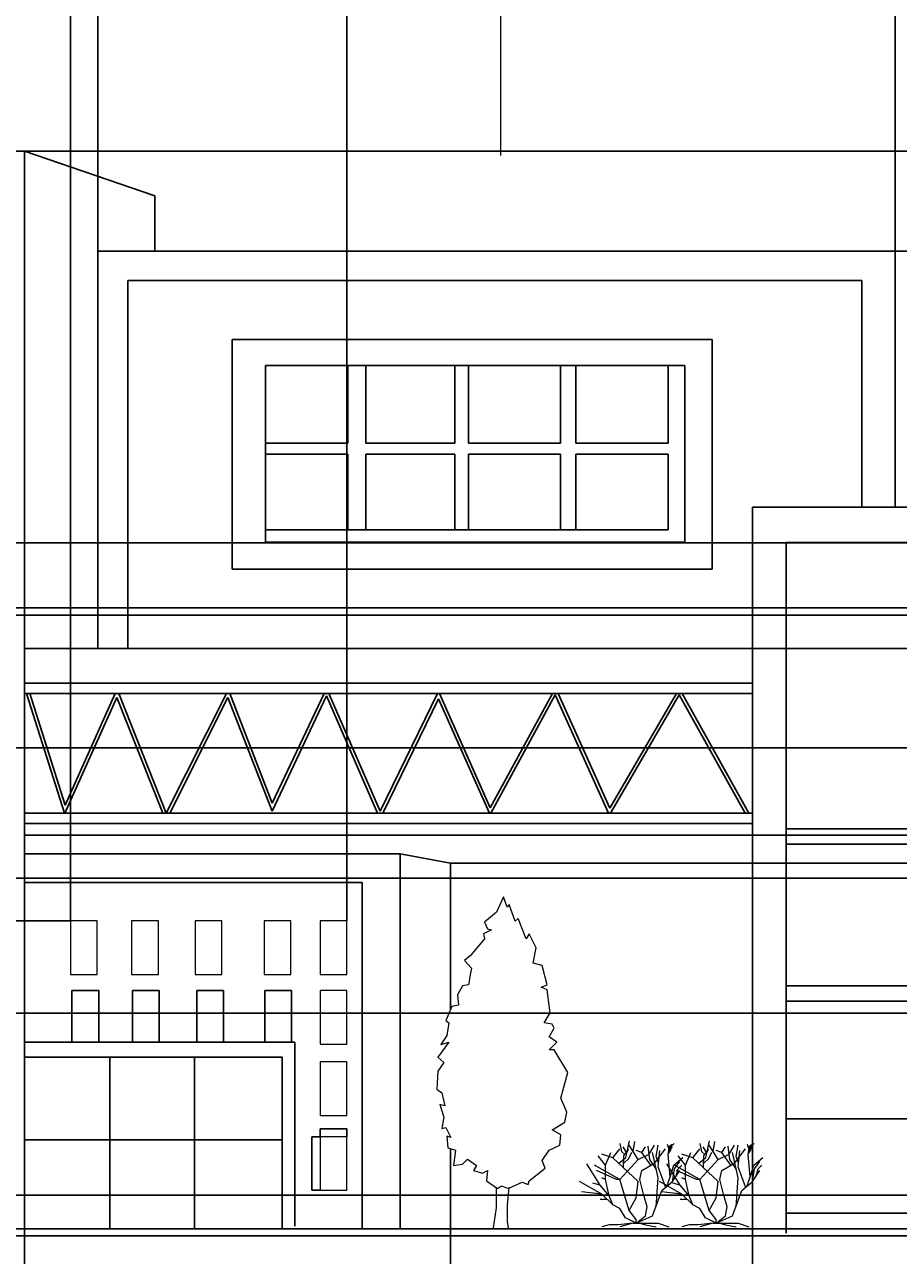
# Model space of a CAD drawing. Units: inches. Extents: x -32109 to 33221, y -19197 to 7608.
# Tile 6 of 25: x -4279 to -741, y -16323 to -11338. Entities that reach past the tile are written whole.
import ezdxf

# ---------------------------------------------------------------- set-up
doc = ezdxf.new("R2010")
doc.units = ezdxf.units.IN
doc.header["$MEASUREMENT"] = 0
for name, color, linetype, lineweight in [('A-ANNO-DIMS', 2, 'Continuous', 18), ('A-ANNO-NOTE', 2, 'Continuous', 18), ('A-ELEV', 7, 'Continuous', 25), ('A-GLAZ', 4, 'Continuous', 18), ('L-PLNT', 3, 'Continuous', 13)]:
    doc.layers.add(name, color=color, linetype=linetype, lineweight=lineweight)
doc.styles.get("Standard").update_dxf_attribs({"font": 'arial.ttf'})
doc.dimstyles.get("Standard").update_dxf_attribs({"dimtxt": 0.18, "dimasz": 0.18, "dimexe": 0.18, "dimexo": 0.0625, "dimgap": 0.09, "dimtad": 0, "dimtih": 1, "dimtoh": 1, "dimdec": 4, "dimzin": 0, "dimdsep": 46, "dimtxsty": 'Standard', "dimcen": 0.09, "dimadec": 0, "dimazin": 0, "dimtfac": 1, "dimtdec": 4, "dimtofl": 0, "dimtmove": 0, "dimatfit": 3, "dimfxl": 1, "dimtolj": 1, "dimtzin": 0, "dimarcsym": 0})

# ---------------------------------------------------------------- blocks, each defined once
blk = doc.blocks.new('*U2')
blk.add_lwpolyline([(-2.754, 191.699), (-6.78, 182.851), (-13.682, 176.953), (-11.956, 173.266), (-9.656, 172.529), (-14.257, 170.317), (-13.682, 167.368), (-21.733, 157.783), (-25.184, 154.834), (-21.158, 150.41), (-21.733, 147.461), (-22.884, 140.825), (-26.334, 140.087), (-29.21, 134.926), (-28.635, 129.028), (-32.661, 128.291), (-36.111, 120.18), (-34.386, 118.706), (-35.536, 111.333), (-38.987, 106.171), (-34.386, 107.646), (-40.712, 98.798), (-37.261, 95.849), (-40.712, 90.688), (-41.287, 80.366), (-38.412, 78.154), (-36.686, 70.781), (-39.562, 71.518), (-37.261, 64.145), (-38.412, 57.509), (-36.111, 58.247), (-33.236, 52.348), (-35.536, 53.086), (-34.961, 46.45), (-30.36, 44.975), (-31.51, 36.128), (-26.334, 36.865), (-23.459, 39.814), (-18.283, 36.128), (-20.008, 33.178), (-14.832, 31.704), (-11.956, 33.178), (-12.531, 27.28), (-6.205, 22.856), (-3.905, 24.331), (0.121, 22.856), (8.173, 26.543), (11.624, 25.068), (12.199, 27.28), (21.4, 34.653), (19.675, 39.077), (23.701, 44.975), (30.027, 47.924), (30.602, 53.823), (25.426, 56.772), (32.903, 61.196), (34.053, 67.094), (30.602, 75.205), (34.628, 89.951), (26.576, 103.222), (23.701, 103.222), (28.302, 107.646), (23.701, 110.595), (26.576, 115.756), (25.426, 117.968), (20.825, 118.706), (24.276, 124.604), (22.551, 137.876), (19.1, 139.35), (22.551, 140.825), (19.675, 151.884), (14.499, 153.359), (16.224, 162.207), (12.199, 170.317), (10.473, 167.368), (5.872, 179.165), (4.147, 177.69), (0.696, 187.275), (-0.454, 185.8)], close=True)
for points in [[(-6.813, 23.669), (-6.813, 11.669), (-8.627, 0)], [(0.387, 23.669), (-0.576, 13.271), (-0.576, 3.686), (0, 0)]]:
    blk.add_lwpolyline(points)
blk = doc.blocks.new('*U3')
for p, q in [((-16.8, 16.32), (-15.36, 19.68)), ((-14.88, 18.24), (-12.96, 20.64)), ((-12.471, 19.775), (-12.898, 22.044)), ((-11.677, 19.071), (-12.471, 19.775)), ((-11.28, 19.619), (-12.104, 21.184)), ((-11.921, 18.836), (-10.64, 20.401)), ((-11.433, 18.289), (-10.457, 22.749)), ((-10.579, 18.054), (-9.846, 19.697)), ((-8.16, 17.76), (-10.56, 21.6)), ((-9.48, 19.775), (-8.992, 22.592)), ((-7.2, 19.68), (-8.64, 20.16)), ((-7.2, 19.68), (-6.24, 21.12)), ((-4.8, 16.32), (-7.2, 19.68)), ((-5.086, 17.741), (-5.513, 21.34)), ((-5.28, 19.2), (-3.84, 21.6)), ((-2.88, 12.96), (-4.32, 19.68)), ((-3.84, 16.8), (-0.96, 20.64)), ((-3.377, 18.602), (-2.888, 21.575)), ((-2.88, 15.84), (-2.4, 20.16)), ((-0.508, 21.888), (-0.081, 20.558)), ((-0.203, 19.149), (0.102, 21.34)), ((-0.142, 19.384), (0.59, 20.401)), ((-0.02, 20.01), (0.896, 21.105)), ((0.041, 20.714), (1.384, 22.044)), ((0.102, 21.34), (0.835, 21.888)), ((-18.24, 11.04), (-21.755, 16.655)), ((-12.96, 12.48), (-19.68, 16.32)), ((-16.8, 16.32), (-18.72, 18.72)), ((-14.88, 18.24), (-17.76, 19.2)), ((-16.8, 12.48), (-16.8, 16.32)), ((-8.16, 12), (-14.88, 18.24)), ((-13.325, 16.724), (-11.433, 18.289)), ((-12.96, 12.48), (-8.16, 17.76)), ((-12.043, 15.628), (-11.921, 18.836)), ((-11.982, 16.802), (-10.579, 18.054)), ((-8.16, 17.76), (-5.28, 19.2)), ((-7.2, 14.88), (-3.84, 16.8)), ((-3.377, 15.315), (-5.086, 17.819)), ((-2.766, 16.802), (-3.377, 18.602)), ((0.346, 13.203), (-0.203, 19.149)), ((1.323, 16.254), (3.642, 18.289)), ((1.44, 15.36), (2.88, 17.28)), ((2.4, 15.36), (3.36, 16.32)), ((-13.92, 12.48), (-19.2, 14.88)), ((-7.68, 12.48), (-7.2, 14.88)), ((-0.96, 10.56), (-2.88, 15.84)), ((-0.48, 10.8), (0.346, 13.203)), ((0.346, 13.203), (1.323, 16.254)), ((0.96, 12), (1.44, 15.36)), ((0.96, 12), (2.88, 14.88)), ((1.92, 13.44), (2.4, 15.36)), ((-17.76, 8.64), (-23.663, 11.961)), ((-18.24, 11.04), (-20.16, 11.52)), ((-15.84, 8.16), (-18.24, 11.04)), ((-16.8, 12.48), (-17.76, 12.96)), ((-15.84, 8.16), (-16.8, 12.48)), ((-12.96, 12.48), (-13.92, 12.48)), ((-10.56, 4.32), (-12.96, 12.48)), ((-8.64, 7.68), (-8.16, 12)), ((-6.72, 8.64), (-7.68, 12.48)), ((-3.36, 5.28), (-2.88, 12.96)), ((-1.92, 9.6), (0.96, 12)), ((-17.76, 8.64), (-23.128, 9.222)), ((-16.32, 7.2), (-18.24, 7.2)), ((-14.88, 5.76), (-17.76, 8.64)), ((-14.88, 5.76), (-15.84, 8.16)), ((-10.56, 4.32), (-8.64, 7.68)), ((-5.76, 5.28), (-6.72, 8.64)), ((-4.32, 2.88), (-1.92, 9.6)), ((-12.96, 4.8), (-14.88, 5.76)), ((-11.52, 2.4), (-12.96, 4.8)), ((-8.64, 1.92), (-10.56, 4.32)), ((-6.24, 2.88), (-5.76, 5.28)), ((-15.84, 0.48), (-17.76, 0)), ((-13.44, 0.48), (-15.84, 0.48)), ((-9.6, 0.96), (-13.44, 0.48)), ((-9.6, 0.96), (-12.96, 0)), ((-8.64, 0.96), (-11.52, 2.4)), ((-9.6, 0.96), (-7.68, 0.96)), ((-8.64, 0.96), (-4.32, 2.88)), ((-8.64, 0.96), (-6.24, 2.88)), ((-8.64, 0.96), (-8.64, 1.92)), ((-8.64, 0.96), (-2.88, 0.96)), ((-7.68, 0.96), (-6.24, 0.48)), ((-6.24, 0.48), (-3.36, 0)), ((-2.88, 0.96), (0, 0))]:
    blk.add_line(p, q)
blk = doc.blocks.new('WIN-SMALL-B')
for p, q in [((0, 216.8), (0, 0)), ((108.5, 216.8), (0, 216.8)), ((108.5, 0), (108.5, 216.8)), ((0, 0), (108.5, 0))]:
    blk.add_line(p, q)
blk = doc.blocks.new('*D8')
at = {"layer": 'A-ANNO-DIMS', "color": 0, "lineweight": -2, "transparency": 16777216}
for p, q in [((-3082.8, -15842.3), (-3115.5, -15842.3)), ((-3115.3, -15842.5), (-3115.3, -15950.5)), ((-3115.3, -16058.9), (-3115.3, -15950.9)), ((-3082.8, -16059.1), (-3115.5, -16059.1))]:
    blk.add_line(p, q, dxfattribs=at)
at = {"layer": 'A-ANNO-DIMS', "color": 0, "transparency": 16777216}
for points in [[(-3115.3, -15842.5), (-3115.3, -15842.5), (-3115.3, -15842.3)], [(-3115.3, -16058.9), (-3115.3, -16058.9), (-3115.3, -16059.1)]]:
    blk.add_solid(points, dxfattribs=at)
at = {"layer": 'Defpoints', "color": 0, "transparency": 16777216}
for p in [(-3115.3, -15842.3), (-3082.8, -15842.3), (-3082.8, -16059.1)]:
    blk.add_point(p, dxfattribs=at)
at = {"layer": 'A-ANNO-DIMS', "color": 0, "transparency": 16777216, "insert": (-3115.3, -15950.7), "char_height": 0.18, "attachment_point": 5}
blk.add_mtext('\\A1;SMALL WINDOW B 217 TYP.', dxfattribs=at)
blk = doc.blocks.new('*D9')
at = {"layer": 'A-ANNO-DIMS', "color": 0, "lineweight": -2, "transparency": 16777216}
for p, q in [((-3082.8, -15842.2), (-3082.8, -15809.6)), ((-3082.6, -15809.8), (-3029.1, -15809.8)), ((-2974.4, -15809.8), (-3027.9, -15809.8)), ((-2974.2, -15842.2), (-2974.2, -15809.6))]:
    blk.add_line(p, q, dxfattribs=at)
at = {"layer": 'A-ANNO-DIMS', "color": 0, "transparency": 16777216}
for points in [[(-3082.6, -15809.7), (-3082.6, -15809.8), (-3082.8, -15809.8)], [(-2974.4, -15809.7), (-2974.4, -15809.8), (-2974.2, -15809.8)]]:
    blk.add_solid(points, dxfattribs=at)
at = {"layer": 'Defpoints', "color": 0, "transparency": 16777216}
for p in [(-3082.8, -15842.3), (-2974.2, -15809.8), (-2974.2, -15842.3)]:
    blk.add_point(p, dxfattribs=at)
at = {"layer": 'A-ANNO-DIMS', "color": 0, "transparency": 16777216, "insert": (-3028.5, -15809.8), "char_height": 0.18, "attachment_point": 5}
blk.add_mtext('\\A1;109 TYP.', dxfattribs=at)
blk = doc.blocks.new('*D13')
at = {"layer": 'A-ANNO-DIMS', "color": 0, "lineweight": -2, "transparency": 16777216}
for p, q in [((-21916.3, -16214.9), (-21916.3, -19197.3)), ((5067.2, -16244.2), (5067.2, -19197.3)), ((-21916.1, -19197.2), (-8425, -19197.2)), ((5067, -19197.2), (-8424.2, -19197.2))]:
    blk.add_line(p, q, dxfattribs=at)
at = {"layer": 'A-ANNO-DIMS', "color": 0, "transparency": 16777216}
for points in [[(-21916.1, -19197.1), (-21916.1, -19197.2), (-21916.3, -19197.2)], [(5067, -19197.1), (5067, -19197.2), (5067.2, -19197.2)]]:
    blk.add_solid(points, dxfattribs=at)
at = {"layer": 'Defpoints', "color": 0, "transparency": 16777216}
for p in [(-21916.3, -16214.8), (5067.2, -16244.1), (5067.2, -19197.2)]:
    blk.add_point(p, dxfattribs=at)
at = {"layer": 'A-ANNO-DIMS', "color": 0, "transparency": 16777216, "insert": (-8424.6, -19197.2), "char_height": 0.18, "attachment_point": 5}
blk.add_mtext('\\A1;26983', dxfattribs=at)
blk = doc.blocks.new('*D14')
at = {"layer": 'A-ANNO-DIMS', "color": 0, "lineweight": -2, "transparency": 16777216}
for p, q in [((-18893.9, -10978.7), (-32108.4, -10978.7)), ((-32108.2, -10978.9), (-32108.2, -13611.2)), ((-32108.2, -16243.9), (-32108.2, -13611.6)), ((5067.1, -16244.1), (-32108.4, -16244.1))]:
    blk.add_line(p, q, dxfattribs=at)
at = {"layer": 'A-ANNO-DIMS', "color": 0, "transparency": 16777216}
for points in [[(-32108.2, -10978.9), (-32108.2, -10978.9), (-32108.2, -10978.7)], [(-32108.2, -16243.9), (-32108.2, -16243.9), (-32108.2, -16244.1)]]:
    blk.add_solid(points, dxfattribs=at)
at = {"layer": 'Defpoints', "color": 0, "transparency": 16777216}
for p in [(-18893.8, -10978.7), (-32108.2, -16244.1), (5067.2, -16244.1)]:
    blk.add_point(p, dxfattribs=at)
at = {"layer": 'A-ANNO-DIMS', "color": 0, "transparency": 16777216, "insert": (-32108.2, -13611.4), "char_height": 0.18, "attachment_point": 5}
blk.add_mtext('\\A1;5265', dxfattribs=at)
blk = doc.blocks.new('*D22')
at = {"layer": 'A-ANNO-DIMS', "color": 0, "lineweight": -2, "transparency": 16777216}
for p, q in [((-4093.7, -14968), (-4093.7, -7335)), ((-4093.5, -7335.2), (-3534.4, -7335.2)), ((-2974.4, -7335.2), (-3533.5, -7335.2)), ((-2974.2, -14968), (-2974.2, -7335))]:
    blk.add_line(p, q, dxfattribs=at)
at = {"layer": 'A-ANNO-DIMS', "color": 0, "transparency": 16777216}
for points in [[(-4093.5, -7335.1), (-4093.5, -7335.2), (-4093.7, -7335.2)], [(-2974.4, -7335.1), (-2974.4, -7335.2), (-2974.2, -7335.2)]]:
    blk.add_solid(points, dxfattribs=at)
at = {"layer": 'Defpoints', "color": 0, "transparency": 16777216}
for p in [(-2974.2, -7335.2), (-4093.7, -14968.1), (-2974.2, -14968.1)]:
    blk.add_point(p, dxfattribs=at)
at = {"layer": 'A-ANNO-DIMS', "color": 0, "transparency": 16777216, "insert": (-3534, -7335.2), "char_height": 0.18, "attachment_point": 5}
blk.add_mtext('\\A1;1119.4', dxfattribs=at)
blk = doc.blocks.new('*D23')
at = {"layer": 'A-ANNO-DIMS', "color": 0, "lineweight": -2, "transparency": 16777216}
for p, q in [((-4093.7, -14968.1), (-32108.4, -14968.1)), ((-32108.2, -14968.3), (-32108.2, -15591.3)), ((-32108.2, -16214.6), (-32108.2, -15591.6)), ((-4279, -16214.8), (-32108.4, -16214.8))]:
    blk.add_line(p, q, dxfattribs=at)
at = {"layer": 'A-ANNO-DIMS', "color": 0, "transparency": 16777216}
for points in [[(-32108.2, -14968.3), (-32108.2, -14968.3), (-32108.2, -14968.1)], [(-32108.2, -16214.6), (-32108.2, -16214.6), (-32108.2, -16214.8)]]:
    blk.add_solid(points, dxfattribs=at)
at = {"layer": 'Defpoints', "color": 0, "transparency": 16777216}
for p in [(-32108.2, -14968.1), (-4093.7, -14968.1), (-4279, -16214.8)]:
    blk.add_point(p, dxfattribs=at)
at = {"layer": 'A-ANNO-DIMS', "color": 0, "transparency": 16777216, "insert": (-32108.2, -15591.4), "char_height": 0.18, "attachment_point": 5}
blk.add_mtext('\\A1;1246.7', dxfattribs=at)
blk = doc.blocks.new('*D92')
at = {"layer": 'A-ANNO-DIMS', "color": 0, "lineweight": -2, "transparency": 16777216}
for p, q in [((-8664.1, -13437.2), (9252.7, -13437.2)), ((9252.5, -13437.4), (9252.5, -14825.8)), ((9252.5, -16214.6), (9252.5, -14826.2)), ((-8664.1, -16214.8), (9252.7, -16214.8))]:
    blk.add_line(p, q, dxfattribs=at)
at = {"layer": 'A-ANNO-DIMS', "color": 0, "transparency": 16777216}
for points in [[(9252.5, -13437.4), (9252.5, -13437.4), (9252.5, -13437.2)], [(9252.5, -16214.6), (9252.5, -16214.6), (9252.5, -16214.8)]]:
    blk.add_solid(points, dxfattribs=at)
at = {"layer": 'Defpoints', "color": 0, "transparency": 16777216}
for p in [(-8664.1, -13437.2), (-8664.1, -16214.8), (9252.5, -16214.8)]:
    blk.add_point(p, dxfattribs=at)
at = {"layer": 'A-ANNO-DIMS', "color": 0, "transparency": 16777216, "insert": (9252.5, -14826), "char_height": 0.18, "attachment_point": 5}
blk.add_mtext('\\A1;2777.6', dxfattribs=at)
blk = doc.blocks.new('*D99')
at = {"layer": 'A-ANNO-DIMS', "color": 0, "lineweight": -2, "transparency": 16777216}
for p, q in [((-9175.1, -13729), (9252.7, -13729)), ((9252.5, -13729.2), (9252.5, -13997.5)), ((9252.5, -14266.2), (9252.5, -13997.9)), ((-9175.1, -14266.4), (9252.7, -14266.4))]:
    blk.add_line(p, q, dxfattribs=at)
at = {"layer": 'A-ANNO-DIMS', "color": 0, "transparency": 16777216}
for points in [[(9252.5, -13729.2), (9252.5, -13729.2), (9252.5, -13729)], [(9252.5, -14266.2), (9252.5, -14266.2), (9252.5, -14266.4)]]:
    blk.add_solid(points, dxfattribs=at)
at = {"layer": 'Defpoints', "color": 0, "transparency": 16777216}
for p in [(-9175.2, -13729), (-9175.2, -14266.4), (9252.5, -14266.4)]:
    blk.add_point(p, dxfattribs=at)
at = {"layer": 'A-ANNO-DIMS', "color": 0, "transparency": 16777216, "insert": (9252.5, -13997.7), "char_height": 0.18, "attachment_point": 5}
blk.add_mtext('\\A1;537.4', dxfattribs=at)
blk = doc.blocks.new('*D100')
at = {"layer": 'A-ANNO-DIMS', "color": 0, "lineweight": -2, "transparency": 16777216}
for p, q in [((-9175.1, -14266.4), (9252.7, -14266.4)), ((9252.5, -14266.6), (9252.5, -14530.6)), ((9252.5, -14794.9), (9252.5, -14530.9)), ((-9175.1, -14795.1), (9252.7, -14795.1))]:
    blk.add_line(p, q, dxfattribs=at)
at = {"layer": 'A-ANNO-DIMS', "color": 0, "transparency": 16777216}
for points in [[(9252.5, -14266.6), (9252.5, -14266.6), (9252.5, -14266.4)], [(9252.5, -14794.9), (9252.5, -14794.9), (9252.5, -14795.1)]]:
    blk.add_solid(points, dxfattribs=at)
at = {"layer": 'Defpoints', "color": 0, "transparency": 16777216}
for p in [(-9175.2, -14266.4), (-9175.2, -14795.1), (9252.5, -14795.1)]:
    blk.add_point(p, dxfattribs=at)
at = {"layer": 'A-ANNO-DIMS', "color": 0, "transparency": 16777216, "insert": (9252.5, -14530.7), "char_height": 0.18, "attachment_point": 5}
blk.add_mtext('\\A1;528.7', dxfattribs=at)
blk = doc.blocks.new('*D101')
at = {"layer": 'A-ANNO-DIMS', "color": 0, "lineweight": -2, "transparency": 16777216}
for p, q in [((-9175.1, -14795.1), (9252.7, -14795.1)), ((9252.5, -14795.3), (9252.5, -15068.4)), ((9252.5, -15341.8), (9252.5, -15068.7)), ((-9175.1, -15342), (9252.7, -15342))]:
    blk.add_line(p, q, dxfattribs=at)
at = {"layer": 'A-ANNO-DIMS', "color": 0, "transparency": 16777216}
for points in [[(9252.5, -14795.3), (9252.5, -14795.3), (9252.5, -14795.1)], [(9252.5, -15341.8), (9252.5, -15341.8), (9252.5, -15342)]]:
    blk.add_solid(points, dxfattribs=at)
at = {"layer": 'Defpoints', "color": 0, "transparency": 16777216}
for p in [(-9175.2, -14795.1), (-9175.2, -15342), (9252.5, -15342)]:
    blk.add_point(p, dxfattribs=at)
at = {"layer": 'A-ANNO-DIMS', "color": 0, "transparency": 16777216, "insert": (9252.5, -15068.6), "char_height": 0.18, "attachment_point": 5}
blk.add_mtext('\\A1;546.9', dxfattribs=at)
blk = doc.blocks.new('*D102')
at = {"layer": 'A-ANNO-DIMS', "color": 0, "lineweight": -2, "transparency": 16777216}
for p, q in [((-9175.1, -15342), (9252.7, -15342)), ((9252.5, -15342.2), (9252.5, -15710.5)), ((9252.5, -16079.1), (9252.5, -15710.8)), ((-9175.1, -16079.3), (9252.7, -16079.3))]:
    blk.add_line(p, q, dxfattribs=at)
at = {"layer": 'A-ANNO-DIMS', "color": 0, "transparency": 16777216}
for points in [[(9252.5, -15342.2), (9252.5, -15342.2), (9252.5, -15342)], [(9252.5, -16079.1), (9252.5, -16079.1), (9252.5, -16079.3)]]:
    blk.add_solid(points, dxfattribs=at)
at = {"layer": 'Defpoints', "color": 0, "transparency": 16777216}
for p in [(-9175.2, -15342), (-9175.2, -16079.3), (9252.5, -16079.3)]:
    blk.add_point(p, dxfattribs=at)
at = {"layer": 'A-ANNO-DIMS', "color": 0, "transparency": 16777216, "insert": (9252.5, -15710.6), "char_height": 0.18, "attachment_point": 5}
blk.add_mtext('\\A1;737.3', dxfattribs=at)
blk = doc.blocks.new('*D104')
at = {"layer": 'A-ANNO-DIMS', "color": 0, "lineweight": -2, "transparency": 16777216}
for p, q in [((-4279, -16214.9), (-4279, -19197.3)), ((-2554.3, -16214.9), (-2554.3, -19197.3)), ((-4278.8, -19197.2), (-3417.1, -19197.2)), ((-2554.5, -19197.2), (-3416.2, -19197.2))]:
    blk.add_line(p, q, dxfattribs=at)
at = {"layer": 'A-ANNO-DIMS', "color": 0, "transparency": 16777216}
for points in [[(-4278.8, -19197.1), (-4278.8, -19197.2), (-4279, -19197.2)], [(-2554.5, -19197.1), (-2554.5, -19197.2), (-2554.3, -19197.2)]]:
    blk.add_solid(points, dxfattribs=at)
at = {"layer": 'Defpoints', "color": 0, "transparency": 16777216}
for p in [(-4279, -16214.8), (-2554.3, -16214.8), (-2554.3, -19197.2)]:
    blk.add_point(p, dxfattribs=at)
at = {"layer": 'A-ANNO-DIMS', "color": 0, "transparency": 16777216, "insert": (-3416.6, -19197.2), "char_height": 0.18, "attachment_point": 5}
blk.add_mtext('\\A1;1724.6', dxfattribs=at)
blk = doc.blocks.new('*D105')
at = {"layer": 'A-ANNO-DIMS', "color": 0, "lineweight": -2, "transparency": 16777216}
for p, q in [((-2554.3, -16214.9), (-2554.3, -19197.3)), ((-1331.3, -16214.9), (-1331.3, -19197.3)), ((-2554.1, -19197.2), (-1943.2, -19197.2)), ((-1331.5, -19197.2), (-1942.5, -19197.2))]:
    blk.add_line(p, q, dxfattribs=at)
at = {"layer": 'A-ANNO-DIMS', "color": 0, "transparency": 16777216}
for points in [[(-2554.1, -19197.1), (-2554.1, -19197.2), (-2554.3, -19197.2)], [(-1331.5, -19197.1), (-1331.5, -19197.2), (-1331.3, -19197.2)]]:
    blk.add_solid(points, dxfattribs=at)
at = {"layer": 'Defpoints', "color": 0, "transparency": 16777216}
for p in [(-2554.3, -16214.8), (-1331.3, -16214.8), (-1331.3, -19197.2)]:
    blk.add_point(p, dxfattribs=at)
at = {"layer": 'A-ANNO-DIMS', "color": 0, "transparency": 16777216, "insert": (-1942.8, -19197.2), "char_height": 0.18, "attachment_point": 5}
blk.add_mtext('\\A1;1223', dxfattribs=at)
blk = doc.blocks.new('*D106')
at = {"layer": 'A-ANNO-DIMS', "color": 0, "lineweight": -2, "transparency": 16777216}
for p, q in [((-1331.3, -16214.9), (-1331.3, -19197.3)), ((2144.2, -16214.9), (2144.2, -19197.3)), ((-1331.1, -19197.2), (406, -19197.2)), ((2144.1, -19197.2), (406.9, -19197.2))]:
    blk.add_line(p, q, dxfattribs=at)
at = {"layer": 'A-ANNO-DIMS', "color": 0, "transparency": 16777216}
for points in [[(-1331.1, -19197.1), (-1331.1, -19197.2), (-1331.3, -19197.2)], [(2144.1, -19197.1), (2144.1, -19197.2), (2144.2, -19197.2)]]:
    blk.add_solid(points, dxfattribs=at)
at = {"layer": 'Defpoints', "color": 0, "transparency": 16777216}
for p in [(-1331.3, -16214.8), (2144.2, -16214.8), (2144.2, -19197.2)]:
    blk.add_point(p, dxfattribs=at)
at = {"layer": 'A-ANNO-DIMS', "color": 0, "transparency": 16777216, "insert": (406.5, -19197.2), "char_height": 0.18, "attachment_point": 5}
blk.add_mtext('\\A1;3475.6', dxfattribs=at)
blk = doc.blocks.new('*D109')
at = {"layer": 'A-ANNO-DIMS', "color": 0, "lineweight": -2, "transparency": 16777216}
for p, q in [((-3982.4, -12255.9), (-3982.4, -7335)), ((-3982.2, -7335.2), (-2368.7, -7335.2)), ((-754.4, -7335.2), (-2368, -7335.2)), ((-754.2, -12255.9), (-754.2, -7335))]:
    blk.add_line(p, q, dxfattribs=at)
at = {"layer": 'A-ANNO-DIMS', "color": 0, "transparency": 16777216}
for points in [[(-3982.2, -7335.1), (-3982.2, -7335.2), (-3982.4, -7335.2)], [(-754.4, -7335.1), (-754.4, -7335.2), (-754.2, -7335.2)]]:
    blk.add_solid(points, dxfattribs=at)
at = {"layer": 'Defpoints', "color": 0, "transparency": 16777216}
for p in [(-754.2, -7335.2), (-3982.4, -12255.9), (-754.2, -12255.9)]:
    blk.add_point(p, dxfattribs=at)
at = {"layer": 'A-ANNO-DIMS', "color": 0, "transparency": 16777216, "insert": (-2368.3, -7335.2), "char_height": 0.18, "attachment_point": 5}
blk.add_mtext('\\A1;3228', dxfattribs=at)
blk = doc.blocks.new('*D110')
at = {"layer": 'A-ANNO-DIMS', "color": 0, "lineweight": -2, "transparency": 16777216}
for p, q in [((-6449.9, -11850.8), (9252.7, -11850.8)), ((9252.5, -11851), (9252.5, -14032.6)), ((9252.5, -16214.6), (9252.5, -14033)), ((-6952.7, -16214.8), (9252.7, -16214.8))]:
    blk.add_line(p, q, dxfattribs=at)
at = {"layer": 'A-ANNO-DIMS', "color": 0, "transparency": 16777216}
for points in [[(9252.5, -11851), (9252.5, -11851), (9252.5, -11850.8)], [(9252.5, -16214.6), (9252.5, -16214.6), (9252.5, -16214.8)]]:
    blk.add_solid(points, dxfattribs=at)
at = {"layer": 'Defpoints', "color": 0, "transparency": 16777216}
for p in [(-6450, -11850.8), (-6952.8, -16214.8), (9252.5, -16214.8)]:
    blk.add_point(p, dxfattribs=at)
at = {"layer": 'A-ANNO-DIMS', "color": 0, "transparency": 16777216, "insert": (9252.5, -14032.8), "char_height": 0.18, "attachment_point": 5}
blk.add_mtext('\\A1;4364', dxfattribs=at)
blk = doc.blocks.new('*D111')
at = {"layer": 'A-ANNO-DIMS', "color": 0, "lineweight": -2, "transparency": 16777216}
for p, q in [((-6954.6, -13699.5), (9252.7, -13699.5)), ((9252.5, -13699.6), (9252.5, -14957)), ((9252.5, -16214.6), (9252.5, -14957.3)), ((-6952.7, -16214.8), (9252.7, -16214.8))]:
    blk.add_line(p, q, dxfattribs=at)
at = {"layer": 'A-ANNO-DIMS', "color": 0, "transparency": 16777216}
for points in [[(9252.5, -13699.6), (9252.5, -13699.6), (9252.5, -13699.5)], [(9252.5, -16214.6), (9252.5, -16214.6), (9252.5, -16214.8)]]:
    blk.add_solid(points, dxfattribs=at)
at = {"layer": 'Defpoints', "color": 0, "transparency": 16777216}
for p in [(-6954.6, -13699.5), (-6952.8, -16214.8), (9252.5, -16214.8)]:
    blk.add_point(p, dxfattribs=at)
at = {"layer": 'A-ANNO-DIMS', "color": 0, "transparency": 16777216, "insert": (9252.5, -14957.1), "char_height": 0.18, "attachment_point": 5}
blk.add_mtext('\\A1;2515.4', dxfattribs=at)
blk = doc.blocks.new('*D112')
at = {"layer": 'A-ANNO-DIMS', "color": 0, "lineweight": -2, "transparency": 16777216}
for p, q in [((-754.2, -12255.9), (9252.7, -12255.9)), ((9252.5, -12256.1), (9252.5, -14235.2)), ((9252.5, -16214.6), (9252.5, -14235.6)), ((-1331.3, -16214.8), (9252.7, -16214.8))]:
    blk.add_line(p, q, dxfattribs=at)
at = {"layer": 'A-ANNO-DIMS', "color": 0, "transparency": 16777216}
for points in [[(9252.5, -12256.1), (9252.5, -12256.1), (9252.5, -12255.9)], [(9252.5, -16214.6), (9252.5, -16214.6), (9252.5, -16214.8)]]:
    blk.add_solid(points, dxfattribs=at)
at = {"layer": 'Defpoints', "color": 0, "transparency": 16777216}
for p in [(-754.2, -12255.9), (-1331.3, -16214.8), (9252.5, -16214.8)]:
    blk.add_point(p, dxfattribs=at)
at = {"layer": 'A-ANNO-DIMS', "color": 0, "transparency": 16777216, "insert": (9252.5, -14235.4), "char_height": 0.18, "attachment_point": 5}
blk.add_mtext('\\A1;3959', dxfattribs=at)
blk = doc.blocks.new('*D114')
at = {"layer": 'A-ANNO-DIMS', "color": 0, "lineweight": -2, "transparency": 16777216}
for p, q in [((-2554.3, -14734.5), (9252.7, -14734.5)), ((9252.5, -14734.7), (9252.5, -15474.5)), ((9252.5, -16214.6), (9252.5, -15474.8)), ((-2554.3, -16214.8), (9252.7, -16214.8))]:
    blk.add_line(p, q, dxfattribs=at)
at = {"layer": 'A-ANNO-DIMS', "color": 0, "transparency": 16777216}
for points in [[(9252.5, -14734.7), (9252.5, -14734.7), (9252.5, -14734.5)], [(9252.5, -16214.6), (9252.5, -16214.6), (9252.5, -16214.8)]]:
    blk.add_solid(points, dxfattribs=at)
at = {"layer": 'Defpoints', "color": 0, "transparency": 16777216}
for p in [(-2554.3, -14734.5), (-2554.3, -16214.8), (9252.5, -16214.8)]:
    blk.add_point(p, dxfattribs=at)
at = {"layer": 'A-ANNO-DIMS', "color": 0, "transparency": 16777216, "insert": (9252.5, -15474.6), "char_height": 0.18, "attachment_point": 5}
blk.add_mtext('\\A1;1480.3', dxfattribs=at)
blk = doc.blocks.new('*D115')
at = {"layer": 'A-ANNO-DIMS', "color": 0, "lineweight": -2, "transparency": 16777216}
for p, q in [((-1331.3, -13865), (9252.7, -13865)), ((9252.5, -13865.2), (9252.5, -14242.4)), ((9252.5, -14619.9), (9252.5, -14242.8)), ((-1331.3, -14620.1), (9252.7, -14620.1))]:
    blk.add_line(p, q, dxfattribs=at)
at = {"layer": 'A-ANNO-DIMS', "color": 0, "transparency": 16777216}
for points in [[(9252.5, -13865.2), (9252.5, -13865.2), (9252.5, -13865)], [(9252.5, -14619.9), (9252.5, -14619.9), (9252.5, -14620.1)]]:
    blk.add_solid(points, dxfattribs=at)
at = {"layer": 'Defpoints', "color": 0, "transparency": 16777216}
for p in [(-1331.3, -13865), (-1331.3, -14620.1), (9252.5, -14620.1)]:
    blk.add_point(p, dxfattribs=at)
at = {"layer": 'A-ANNO-DIMS', "color": 0, "transparency": 16777216, "insert": (9252.5, -14242.6), "char_height": 0.18, "attachment_point": 5}
blk.add_mtext('\\A1;755.1', dxfattribs=at)

msp = doc.modelspace()

# ---------------------------------------------------------------- linework, layer by layer
at = {"layer": 'A-ANNO-NOTE'}
msp.add_line((-2350.305, -11867.634), (-2350.305, -9225.16), dxfattribs=at)
at = {"layer": 'A-ELEV'}
for p, q in [((-4278.952, -11850.794), (-6449.955, -11850.794)), ((-4278.952, -12597.537), (-4278.952, -11850.794)), ((-4278.952, -11850.794), (-3751.65, -12030.946)), ((-3751.65, -12255.932), (-3751.65, -12030.946)), ((-3982.394, -12255.932), (-754.237, -12255.932)), ((-3982.394, -12255.932), (-3982.394, -13865.048)), ((-754.237, -12255.932), (-754.237, -13292.138)), ((-3861.02, -13865.048), (-3861.02, -12374.268)), ((-3861.02, -12374.268), (-888.646, -12374.268)), ((-888.646, -12374.268), (-888.646, -13292.138)), ((-4278.952, -12597.537), (-4278.952, -13351.579)), ((-3438.285, -12613.616), (-1495.38, -12613.616)), ((-3438.285, -12613.616), (-3438.285, -13542.796)), ((-1495.38, -12613.616), (-1495.38, -13542.796)), ((-3303.775, -12717.852), (-1605.996, -12717.852)), ((-3303.775, -13434.017), (-3303.775, -12717.852)), ((-2969.689, -13033.246), (-2969.689, -12717.852)), ((-2897.083, -13033.246), (-2897.083, -12717.852)), ((-2536.128, -13033.246), (-2536.128, -12717.852)), ((-2481.829, -13033.246), (-2481.829, -12717.852)), ((-2108.79, -13033.246), (-2108.79, -12717.852)), ((-2046.71, -13033.246), (-2046.71, -12717.852)), ((-1673.154, -13033.246), (-1673.154, -12717.852)), ((-1605.996, -12717.852), (-1605.996, -13434.017)), ((-3303.775, -13033.246), (-2969.689, -13033.246)), ((-2897.083, -13033.246), (-2536.128, -13033.246)), ((-2481.829, -13033.246), (-2108.79, -13033.246)), ((-2046.71, -13033.246), (-1673.154, -13033.246)), ((-3303.775, -13077.73), (-2969.689, -13077.73)), ((-2969.689, -13383.888), (-2969.689, -13077.73)), ((-2897.083, -13383.888), (-2897.083, -13077.73)), ((-2897.083, -13077.73), (-2536.128, -13077.73)), ((-2536.128, -13383.888), (-2536.128, -13077.73)), ((-2481.829, -13383.888), (-2481.829, -13077.73)), ((-2481.829, -13077.73), (-2108.79, -13077.73)), ((-2108.79, -13383.888), (-2108.79, -13077.73)), ((-2046.71, -13383.888), (-2046.71, -13077.73)), ((-2046.71, -13077.73), (-1673.154, -13077.73)), ((-1673.154, -13383.888), (-1673.154, -13077.73)), ((-1331.314, -13292.138), (-1331.314, -16214.811)), ((-1331.314, -13292.138), (2144.248, -13292.138)), ((-4278.952, -13924.489), (-4278.952, -13351.579)), ((-3303.775, -13383.888), (-1673.154, -13383.888)), ((-1605.996, -13434.017), (-3303.775, -13434.017)), ((-1195.362, -16232.478), (-1195.362, -13434.772)), ((-1195.362, -13434.772), (1987.069, -13434.772)), ((-3438.285, -13542.796), (-1495.38, -13542.796)), ((-1331.314, -13865.048), (-4278.952, -13865.048)), ((-4278.952, -13924.489), (-4278.952, -14561.051)), ((-4278.952, -14000.151), (-4278.952, -16214.811)), ((-1331.314, -14004.944), (-4278.952, -14004.944)), ((-4278.952, -14046.764), (-4278.952, -14004.944)), ((-1331.314, -14046.764), (-4278.952, -14046.764)), ((-4117.932, -14531.857), (-4271.842, -14046.891)), ((-4115.108, -14498.509), (-4258.475, -14046.764)), ((-3912.102, -14046.764), (-4115.108, -14498.509)), ((-3705.09, -14531.857), (-3897.938, -14046.423)), ((-3462.035, -14046.764), (-3705.09, -14531.857)), ((-3275.83, -14491.639), (-3448.329, -14046.764)), ((-3056.677, -14056.801), (-3276.975, -14524.034)), ((-3066.073, -14046.764), (-3275.83, -14491.639)), ((-2849.282, -14531.857), (-3056.677, -14056.801)), ((-2838.753, -14524.034), (-3047.114, -14046.764)), ((-2606.737, -14046.764), (-2838.753, -14524.034)), ((-2393.036, -14509.333), (-2599.166, -14046.764)), ((-2141.396, -14046.764), (-2393.036, -14509.333)), ((-2130.095, -14052.733), (-2390.741, -14531.857)), ((-1914.562, -14531.208), (-2130.095, -14052.733)), ((-1909.364, -14511.633), (-2118.768, -14046.764)), ((-1639.101, -14046.764), (-1909.364, -14511.633)), ((-1627.728, -14052.628), (-1906.339, -14531.857)), ((-1360.427, -14531.857), (-1627.728, -14052.628)), ((-1345.794, -14531.857), (-1616.365, -14046.764)), ((-3905.237, -14062.665), (-4116.084, -14531.857)), ((-3718.841, -14531.857), (-3905.237, -14062.665)), ((-3455.799, -14062.846), (-3690.796, -14531.857)), ((-3276.975, -14524.034), (-3455.799, -14062.846)), ((-2603.291, -14068.905), (-2828.346, -14531.857)), ((-2398.158, -14529.236), (-2603.291, -14068.905)), ((-4237.321, -14531.857), (-4278.952, -14531.857)), ((-1331.314, -14531.857), (-4237.321, -14531.857)), ((-4237.321, -14573.061), (-4278.952, -14573.061)), ((-4237.321, -14573.061), (-1331.314, -14573.061)), ((-1195.362, -14595.055), (1987.069, -14595.055)), ((-1331.314, -14620.13), (-4278.952, -14620.13)), ((-4278.952, -14695.733), (-2758.492, -14695.733)), ((-2758.492, -14695.733), (-2758.492, -16214.811)), ((-2758.492, -14695.733), (-2554.321, -14734.483)), ((-1195.362, -14656.763), (1987.069, -14656.763)), ((-2554.321, -14734.483), (-2554.321, -15325.263)), ((-2912.708, -14812.109), (-4278.952, -14812.109)), ((-2912.708, -16214.811), (-2912.708, -14812.109)), ((-4087.527, -15249.927), (-4087.527, -15458.484)), ((-3978.994, -15249.927), (-4087.527, -15249.927)), ((-3978.994, -15458.484), (-3978.994, -15249.927)), ((-3842.552, -15249.927), (-3842.552, -15458.484)), ((-3734.019, -15249.927), (-3842.552, -15249.927)), ((-3734.019, -15458.484), (-3734.019, -15249.927)), ((-3582.073, -15249.927), (-3582.073, -15458.484)), ((-3473.54, -15249.927), (-3582.073, -15249.927)), ((-3473.54, -15458.484), (-3473.54, -15249.927)), ((-3306.089, -15249.927), (-3306.089, -15458.484)), ((-3197.556, -15249.927), (-3306.089, -15249.927)), ((-3197.556, -15458.484), (-3197.556, -15249.927)), ((-1195.362, -15231.592), (1987.069, -15231.592)), ((-1195.362, -15293.299), (1987.069, -15293.299)), ((-3184.72, -15458.484), (-4278.952, -15458.484)), ((-3184.72, -16204.18), (-3184.72, -15458.484)), ((-3236.429, -15519.49), (-4278.952, -15519.49)), ((-3933.341, -15519.49), (-3933.341, -16214.811)), ((-3590.753, -15519.49), (-3590.753, -16214.811)), ((-3236.429, -16214.811), (-3236.429, -15519.49)), ((-1195.362, -15769.96), (1456.232, -15769.96)), ((-2554.321, -15843.911), (-2554.321, -15845.165)), ((-3236.429, -15854.686), (-4278.952, -15854.686)), ((-2554.321, -15890.296), (-2554.321, -16214.811)), ((-1195.362, -16151.095), (1987.069, -16151.095)), ((-12087.226, -16214.811), (7362.494, -16214.811)), ((-1417.009, -16214.811), (-10157.643, -16214.811)), ((-4278.952, -16214.811), (-4355.795, -16214.811)), ((-2758.492, -16214.811), (-2912.708, -16214.811))]:
    msp.add_line(p, q, dxfattribs=at)

# ---------------------------------------------------------------- block references
at = {"layer": 'A-GLAZ'}
for p in [(-4093.675, -15184.885), (-3845.6, -15184.885), (-3588.221, -15184.885), (-3309.137, -15184.885), (-3082.768, -15184.885), (-3082.768, -15466.733), (-3082.768, -15755.563), (-3082.768, -16059.092)]:
    msp.add_blockref('WIN-SMALL-B', p, dxfattribs=at)
at = {"layer": 'L-PLNT'}
for name, p, xscale, yscale, zscale in [('*U2', (-2321.079, -16211.622), 6.995961062916478, 6.995961062916478, 6.995961062916478), ('*U3', (-1669.59, -16206.683), 15.30854395898754, 15.30854395898754, 15.30854395898754), ('*U3', (-1345.612, -16206.683), 15.30854395898754, 15.30854395898754, 15.30854395898754)]:
    msp.add_blockref(name, p, dxfattribs=dict(at, xscale=xscale, yscale=yscale, zscale=zscale))

# ---------------------------------------------------------------- dimensions: what is measured, and where the dimension line sits
at = {"layer": 'A-ANNO-DIMS'}
for base, p1, p2, override, picture, middle in [((-2974.235, -7335.16), (-4093.675, -14968.079), (-2974.235, -14968.079), {"dimdec": 1, "dimlfac": 1, "dimrnd": 0, "dimzin": 0, "dimdsep": 46, "dimlunit": 2}, '*D22', (-3533.955, -7335.16)), ((-754.237, -7335.16), (-3982.394, -12255.932), (-754.237, -12255.932), {"dimdec": 0, "dimlfac": 1, "dimrnd": 0, "dimzin": 0, "dimdsep": 46, "dimlunit": 2}, '*D109', (-2368.316, -7335.16)), ((5067.151, -19197.169), (-21916.328, -16214.811), (5067.151, -16244.113), {"dimdec": 0, "dimlfac": 1, "dimrnd": 0, "dimzin": 0, "dimdsep": 46, "dimlunit": 2}, '*D13', (-8424.588, -19197.169)), ((-2554.321, -19197.169), (-4278.952, -16214.811), (-2554.321, -16214.811), {"dimdec": 1, "dimlfac": 1, "dimrnd": 0, "dimzin": 0, "dimdsep": 46, "dimlunit": 2}, '*D104', (-3416.636, -19197.169)), ((-1331.314, -19197.169), (-2554.321, -16214.811), (-1331.314, -16214.811), {"dimdec": 0, "dimlfac": 1, "dimrnd": 0, "dimzin": 0, "dimdsep": 46, "dimlunit": 2}, '*D105', (-1942.818, -19197.169)), ((2144.248, -19197.169), (-1331.314, -16214.811), (2144.248, -16214.811), {"dimdec": 1, "dimlfac": 1, "dimrnd": 0, "dimzin": 0, "dimdsep": 46, "dimlunit": 2}, '*D106', (406.467, -19197.169))]:
    dim = msp.add_linear_dim(base=base, p1=p1, p2=p2, dimstyle='Standard', override=override, dxfattribs=at)
    dim.commit()
    dim.dimension.update_dxf_attribs({"geometry": picture, "text_midpoint": middle})
for base, p1, p2, override, picture, middle in [((-32108.187, -16244.113), (-18893.845, -10978.73), (5067.151, -16244.113), {"dimdec": 0, "dimlfac": 1, "dimrnd": 0, "dimzin": 0, "dimdsep": 46, "dimlunit": 2}, '*D14', (-32108.187, -13611.422)), ((9252.494, -16214.811), (-6449.955, -11850.794), (-6952.774, -16214.811), {"dimdec": 0, "dimlfac": 1, "dimrnd": 0, "dimzin": 0, "dimdsep": 46, "dimlunit": 2}, '*D110', (9252.494, -14032.802)), ((9252.494, -16214.811), (-754.237, -12255.932), (-1331.314, -16214.811), {"dimdec": 0, "dimlfac": 1, "dimrnd": 0, "dimzin": 0, "dimdsep": 46, "dimlunit": 2}, '*D112', (9252.494, -14235.371)), ((9252.494, -16214.811), (-8664.143, -13437.203), (-8664.143, -16214.811), {"dimdec": 1, "dimlfac": 1, "dimrnd": 0, "dimzin": 0, "dimdsep": 46, "dimlunit": 2}, '*D92', (9252.494, -14826.007)), ((9252.494, -16214.811), (-6954.623, -13699.459), (-6952.774, -16214.811), {"dimdec": 1, "dimlfac": 1, "dimrnd": 0, "dimzin": 0, "dimdsep": 46, "dimlunit": 2}, '*D111', (9252.494, -14957.135)), ((9252.494, -14266.38), (-9175.157, -13729.028), (-9175.157, -14266.38), {"dimdec": 1, "dimlfac": 1, "dimrnd": 0, "dimzin": 0, "dimdsep": 46, "dimlunit": 2}, '*D99', (9252.494, -13997.704)), ((9252.494, -14620.13), (-1331.314, -13865.048), (-1331.314, -14620.13), {"dimdec": 1, "dimlfac": 1, "dimrnd": 0, "dimzin": 0, "dimdsep": 46, "dimlunit": 2}, '*D115', (9252.494, -14242.589)), ((9252.494, -14795.117), (-9175.157, -14266.38), (-9175.157, -14795.117), {"dimdec": 1, "dimlfac": 1, "dimrnd": 0, "dimzin": 0, "dimdsep": 46, "dimlunit": 2}, '*D100', (9252.494, -14530.748)), ((9252.494, -16214.811), (-2554.321, -14734.483), (-2554.321, -16214.811), {"dimdec": 1, "dimlfac": 1, "dimrnd": 0, "dimzin": 0, "dimdsep": 46, "dimlunit": 2}, '*D114', (9252.494, -15474.647)), ((9252.494, -15341.992), (-9175.157, -14795.117), (-9175.157, -15341.992), {"dimdec": 1, "dimlfac": 1, "dimrnd": 0, "dimzin": 0, "dimdsep": 46, "dimlunit": 2}, '*D101', (9252.494, -15068.555)), ((-32108.187, -14968.079), (-4278.952, -16214.811), (-4093.675, -14968.079), {"dimdec": 1, "dimlfac": 1, "dimrnd": 0, "dimzin": 0, "dimdsep": 46, "dimlunit": 2}, '*D23', (-32108.187, -15591.445)), ((9252.494, -16079.3), (-9175.157, -15341.992), (-9175.157, -16079.3), {"dimdec": 1, "dimlfac": 1, "dimrnd": 0, "dimzin": 0, "dimdsep": 46, "dimlunit": 2}, '*D102', (9252.494, -15710.646))]:
    dim = msp.add_linear_dim(base=base, p1=p1, p2=p2, angle=90, dimstyle='Standard', override=override, dxfattribs=at)
    dim.commit()
    dim.dimension.update_dxf_attribs({"geometry": picture, "text_midpoint": middle})
dim = msp.add_linear_dim(base=(-3115.289, -15842.286), p1=(-3082.768, -16059.092), p2=(-3082.768, -15842.286), angle=90, text='SMALL WINDOW B <> TYP.', dimstyle='Standard', override={"dimdec": 0, "dimlfac": 1, "dimrnd": 0, "dimzin": 0, "dimdsep": 46, "dimlunit": 2}, dxfattribs=at)
dim.commit()
dim.dimension.update_dxf_attribs({"geometry": '*D8', "text_midpoint": (-3115.289, -15950.689)})
dim = msp.add_linear_dim(base=(-2974.235, -15809.765), p1=(-3082.768, -15842.286), p2=(-2974.235, -15842.286), text='<> TYP.', dimstyle='Standard', override={"dimdec": 0, "dimlfac": 1, "dimrnd": 0, "dimzin": 0, "dimdsep": 46, "dimlunit": 2}, dxfattribs=at)
dim.commit()
dim.dimension.update_dxf_attribs({"geometry": '*D9', "text_midpoint": (-3028.502, -15809.765)})

doc.saveas('drawing.dxf')
